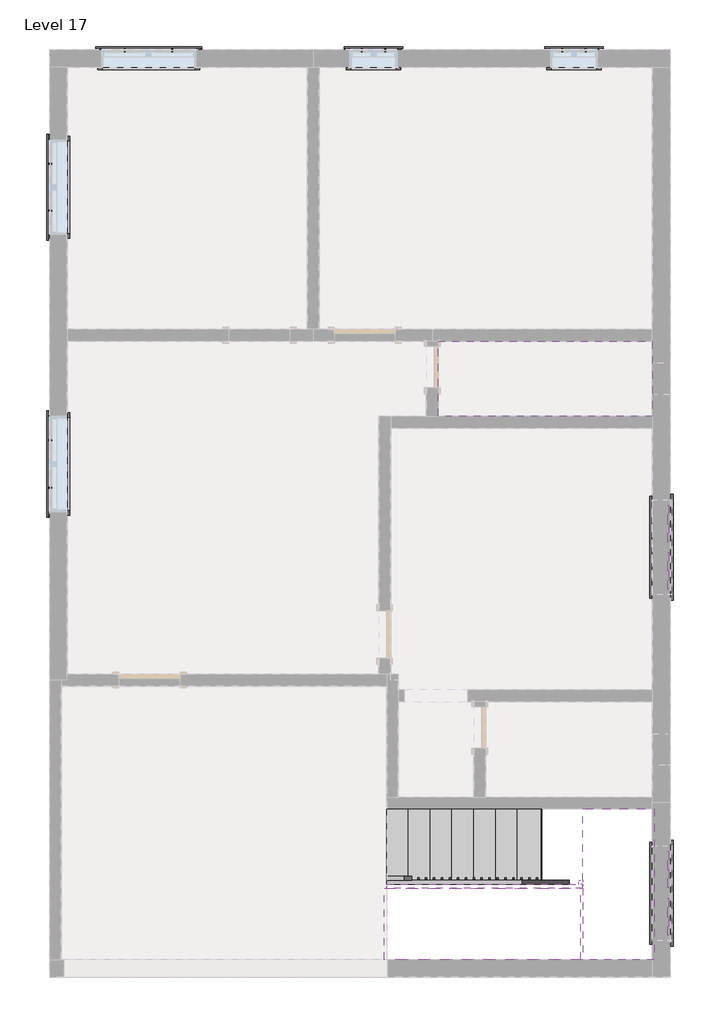
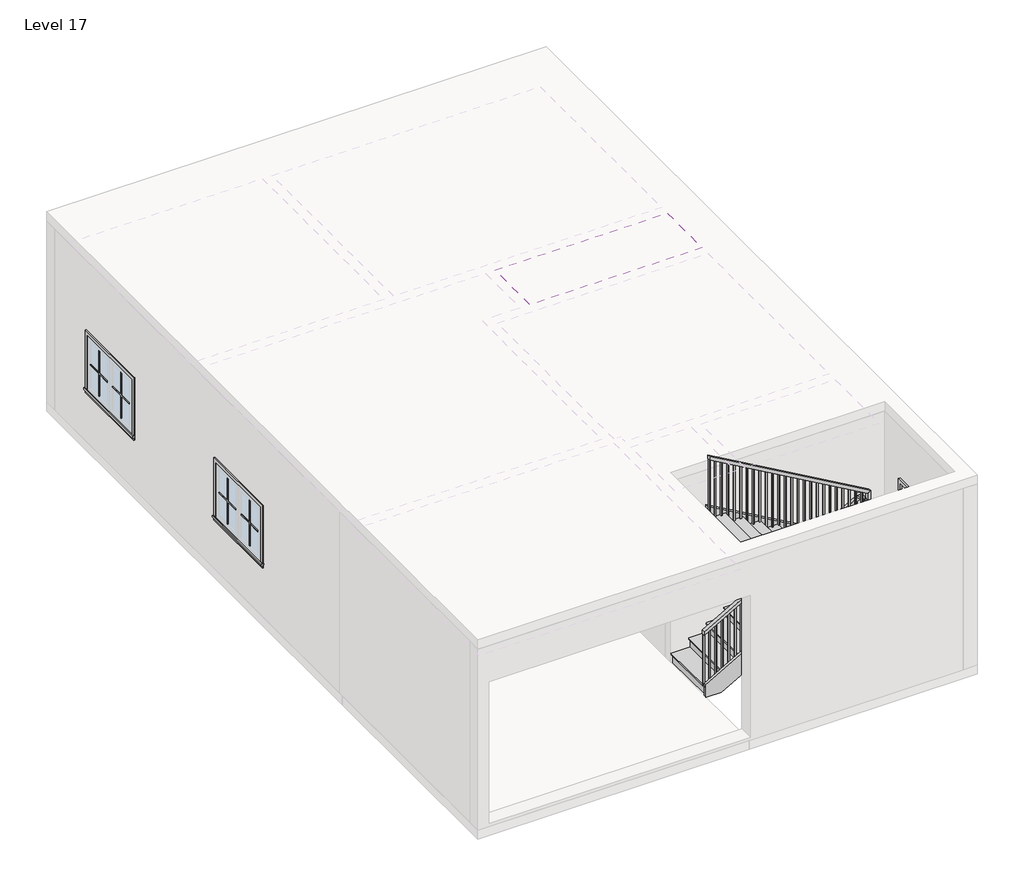
# One storey, part 2 of 2: 44 proxies, 3 members, 2 stair flights, 1 covering, 1 railing, 1 slab.
"""IFC4 building model written with IfcOpenShell, lengths in millimetres."""

from ifc_helpers import new_model, si_unit, frame, origin, place, context, project, spatial, polyline, outline, extrude, faceted_brep, transform, mapped, element, save
from components import muntin_pattern_2x2_muntin_pattern_2x2_2357e71d, muntin_pattern_2x2_muntin_pattern_2x2_302d8f29, muntin_pattern_2x2_muntin_pattern_2x2_53152e2c, muntin_pattern_2x2_muntin_pattern_2x2_e8f3e573, trim_window_exterior_flat_with_sill_c4e67c73, trim_window_exterior_flat_with_sill_a665a915, trim_window_interior_flat_picture_frame_cf1733af, trim_window_interior_flat_picture_frame_d485c387, non_monolithic_landing_9ec975f3, stair_flight_228e22e8, stair_flight_e10c2242

model = new_model("IFC4")

# Units and contexts
model_context = context("Model", 3, world=origin())
ifc_project = project(units=[si_unit("LENGTHUNIT", "METRE", prefix="MILLI")], contexts=[model_context])

# Site, building, storey
site = spatial("IfcSite", under=ifc_project)
building = spatial("IfcBuilding", under=site)
storey = spatial("IfcBuildingStorey", under=building, Name="Level 17", Elevation=9601.2)

# Proxies
placement = place(None, origin())
muntin_pattern_2x2_muntin_pattern_2x2_shape = muntin_pattern_2x2_muntin_pattern_2x2_2357e71d(model_context)
element("IfcBuildingElementProxy", 1, Name="Muntin Pattern_2x2 : Muntin Pattern_2x2", ObjectType="Muntin Pattern_2x2 : Muntin Pattern_2x2", at=placement, inside=storey, context=model_context, shape_type="MappedRepresentation", body=[
    mapped(muntin_pattern_2x2_muntin_pattern_2x2_shape, transform((-4942.3279463, 5897.3080275, 10585.45), x_axis=(1.0, 0.0, 0.0), y_axis=(0.0, 1.0, 0.0), z_axis=(0.0, 0.0, 1.0))),
])
element("IfcBuildingElementProxy", 2, Name="Muntin Pattern_2x2 : Muntin Pattern_2x2", ObjectType="Muntin Pattern_2x2 : Muntin Pattern_2x2", at=placement, inside=storey, context=model_context, shape_type="MappedRepresentation", body=[
    mapped(muntin_pattern_2x2_muntin_pattern_2x2_shape, transform((-5899.5904463, 3838.3205275, 10585.45), x_axis=(0.0, 1.0, 0.0), y_axis=(-1.0, 0.0, 0.0), z_axis=(0.0, 0.0, 1.0))),
])
element("IfcBuildingElementProxy", 3, Name="Muntin Pattern_2x2 : Muntin Pattern_2x2", ObjectType="Muntin Pattern_2x2 : Muntin Pattern_2x2", at=placement, inside=storey, context=model_context, shape_type="MappedRepresentation", body=[
    mapped(muntin_pattern_2x2_muntin_pattern_2x2_shape, transform((-5899.5904463, 293.4330275, 10585.45), x_axis=(0.0, 1.0, 0.0), y_axis=(-1.0, 0.0, 0.0), z_axis=(0.0, 0.0, 1.0))),
])
element("IfcBuildingElementProxy", 4, Name="Muntin Pattern_2x2 : Muntin Pattern_2x2", ObjectType="Muntin Pattern_2x2 : Muntin Pattern_2x2", at=placement, inside=storey, context=model_context, shape_type="MappedRepresentation", body=[
    mapped(muntin_pattern_2x2_muntin_pattern_2x2_shape, transform((2031.5595537, -166.9419725, 10890.25), x_axis=(0.0, -1.0, 0.0), y_axis=(1.0, 0.0, 0.0), z_axis=(0.0, 0.0, 1.0))),
])
element("IfcBuildingElementProxy", 5, Name="Muntin Pattern_2x2 : Muntin Pattern_2x2", ObjectType="Muntin Pattern_2x2 : Muntin Pattern_2x2", at=placement, inside=storey, context=model_context, shape_type="MappedRepresentation", body=[
    mapped(muntin_pattern_2x2_muntin_pattern_2x2_shape, transform((2031.5595537, -4599.2419725, 10890.25), x_axis=(0.0, -1.0, 0.0), y_axis=(1.0, 0.0, 0.0), z_axis=(0.0, 0.0, 1.0))),
])
element("IfcBuildingElementProxy", 6, Name="Muntin Pattern_2x2 : Muntin Pattern_2x2", ObjectType="Muntin Pattern_2x2 : Muntin Pattern_2x2", at=placement, inside=storey, context=model_context, shape_type="MappedRepresentation", body=[
    mapped(muntin_pattern_2x2_muntin_pattern_2x2_shape, transform((-4942.3279463, 5897.3080275, 10585.45), x_axis=(1.0, 0.0, 0.0), y_axis=(0.0, 1.0, 0.0), z_axis=(0.0, 0.0, 1.0))),
])
element("IfcBuildingElementProxy", 7, Name="Muntin Pattern_2x2 : Muntin Pattern_2x2", ObjectType="Muntin Pattern_2x2 : Muntin Pattern_2x2", at=placement, inside=storey, context=model_context, shape_type="MappedRepresentation", body=[
    mapped(muntin_pattern_2x2_muntin_pattern_2x2_shape, transform((2031.5595537, -4599.2419725, 10890.25), x_axis=(0.0, -1.0, 0.0), y_axis=(1.0, 0.0, 0.0), z_axis=(0.0, 0.0, 1.0))),
])
muntin_pattern_2x2_muntin_pattern_2x2_2_shape = muntin_pattern_2x2_muntin_pattern_2x2_302d8f29(model_context)
element("IfcBuildingElementProxy", 8, Name="Muntin Pattern_2x2 : Muntin Pattern_2x2", ObjectType="Muntin Pattern_2x2 : Muntin Pattern_2x2", at=placement, inside=storey, context=model_context, shape_type="MappedRepresentation", body=[
    mapped(muntin_pattern_2x2_muntin_pattern_2x2_2_shape, transform((-4335.9029463, 5897.3080275, 10585.45), x_axis=(-1.0, 0.0, 0.0), y_axis=(0.0, -1.0, 0.0), z_axis=(0.0, 0.0, 1.0))),
])
element("IfcBuildingElementProxy", 9, Name="Muntin Pattern_2x2 : Muntin Pattern_2x2", ObjectType="Muntin Pattern_2x2 : Muntin Pattern_2x2", at=placement, inside=storey, context=model_context, shape_type="MappedRepresentation", body=[
    mapped(muntin_pattern_2x2_muntin_pattern_2x2_2_shape, transform((-5899.5904463, 4444.7455275, 10585.45), x_axis=(0.0, -1.0, 0.0), y_axis=(1.0, 0.0, 0.0), z_axis=(0.0, 0.0, 1.0))),
])
element("IfcBuildingElementProxy", 10, Name="Muntin Pattern_2x2 : Muntin Pattern_2x2", ObjectType="Muntin Pattern_2x2 : Muntin Pattern_2x2", at=placement, inside=storey, context=model_context, shape_type="MappedRepresentation", body=[
    mapped(muntin_pattern_2x2_muntin_pattern_2x2_2_shape, transform((-5899.5904463, 899.8580275, 10585.45), x_axis=(0.0, -1.0, 0.0), y_axis=(1.0, 0.0, 0.0), z_axis=(0.0, 0.0, 1.0))),
])
element("IfcBuildingElementProxy", 11, Name="Muntin Pattern_2x2 : Muntin Pattern_2x2", ObjectType="Muntin Pattern_2x2 : Muntin Pattern_2x2", at=placement, inside=storey, context=model_context, shape_type="MappedRepresentation", body=[
    mapped(muntin_pattern_2x2_muntin_pattern_2x2_2_shape, transform((2031.5595537, -773.3669725, 10890.25), x_axis=(0.0, 1.0, 0.0), y_axis=(-1.0, 0.0, 0.0), z_axis=(0.0, 0.0, 1.0))),
])
element("IfcBuildingElementProxy", 12, Name="Muntin Pattern_2x2 : Muntin Pattern_2x2", ObjectType="Muntin Pattern_2x2 : Muntin Pattern_2x2", at=placement, inside=storey, context=model_context, shape_type="MappedRepresentation", body=[
    mapped(muntin_pattern_2x2_muntin_pattern_2x2_2_shape, transform((2031.5595537, -5205.6669725, 10890.25), x_axis=(0.0, 1.0, 0.0), y_axis=(-1.0, 0.0, 0.0), z_axis=(0.0, 0.0, 1.0))),
])
element("IfcBuildingElementProxy", 13, Name="Muntin Pattern_2x2 : Muntin Pattern_2x2", ObjectType="Muntin Pattern_2x2 : Muntin Pattern_2x2", at=placement, inside=storey, context=model_context, shape_type="MappedRepresentation", body=[
    mapped(muntin_pattern_2x2_muntin_pattern_2x2_2_shape, transform((-4335.9029463, 5897.3080275, 10585.45), x_axis=(-1.0, 0.0, 0.0), y_axis=(0.0, -1.0, 0.0), z_axis=(0.0, 0.0, 1.0))),
])
element("IfcBuildingElementProxy", 14, Name="Muntin Pattern_2x2 : Muntin Pattern_2x2", ObjectType="Muntin Pattern_2x2 : Muntin Pattern_2x2", at=placement, inside=storey, context=model_context, shape_type="MappedRepresentation", body=[
    mapped(muntin_pattern_2x2_muntin_pattern_2x2_2_shape, transform((2031.5595537, -5205.6669725, 10890.25), x_axis=(0.0, 1.0, 0.0), y_axis=(-1.0, 0.0, 0.0), z_axis=(0.0, 0.0, 1.0))),
])
muntin_pattern_2x2_muntin_pattern_2x2_3_shape = muntin_pattern_2x2_muntin_pattern_2x2_53152e2c(model_context)
element("IfcBuildingElementProxy", 15, Name="Muntin Pattern_2x2 : Muntin Pattern_2x2", ObjectType="Muntin Pattern_2x2 : Muntin Pattern_2x2", at=placement, inside=storey, context=model_context, shape_type="MappedRepresentation", body=[
    mapped(muntin_pattern_2x2_muntin_pattern_2x2_3_shape, transform((-1907.0279463, 5897.3080275, 10585.45), x_axis=(1.0, 0.0, 0.0), y_axis=(0.0, 1.0, 0.0), z_axis=(0.0, 0.0, 1.0))),
])
element("IfcBuildingElementProxy", 16, Name="Muntin Pattern_2x2 : Muntin Pattern_2x2", ObjectType="Muntin Pattern_2x2 : Muntin Pattern_2x2", at=placement, inside=storey, context=model_context, shape_type="MappedRepresentation", body=[
    mapped(muntin_pattern_2x2_muntin_pattern_2x2_3_shape, transform((658.3720537, 5897.3080275, 10585.45), x_axis=(1.0, 0.0, 0.0), y_axis=(0.0, 1.0, 0.0), z_axis=(0.0, 0.0, 1.0))),
])
element("IfcBuildingElementProxy", 17, Name="Muntin Pattern_2x2 : Muntin Pattern_2x2", ObjectType="Muntin Pattern_2x2 : Muntin Pattern_2x2", at=placement, inside=storey, context=model_context, shape_type="MappedRepresentation", body=[
    mapped(muntin_pattern_2x2_muntin_pattern_2x2_3_shape, transform((-1907.0279463, 5897.3080275, 10585.45), x_axis=(1.0, 0.0, 0.0), y_axis=(0.0, 1.0, 0.0), z_axis=(0.0, 0.0, 1.0))),
])
element("IfcBuildingElementProxy", 18, Name="Muntin Pattern_2x2 : Muntin Pattern_2x2", ObjectType="Muntin Pattern_2x2 : Muntin Pattern_2x2", at=placement, inside=storey, context=model_context, shape_type="MappedRepresentation", body=[
    mapped(muntin_pattern_2x2_muntin_pattern_2x2_3_shape, transform((658.3720537, 5897.3080275, 10585.45), x_axis=(1.0, 0.0, 0.0), y_axis=(0.0, 1.0, 0.0), z_axis=(0.0, 0.0, 1.0))),
])
muntin_pattern_2x2_muntin_pattern_2x2_4_shape = muntin_pattern_2x2_muntin_pattern_2x2_e8f3e573(model_context)
element("IfcBuildingElementProxy", 19, Name="Muntin Pattern_2x2 : Muntin Pattern_2x2", ObjectType="Muntin Pattern_2x2 : Muntin Pattern_2x2", at=placement, inside=storey, context=model_context, shape_type="MappedRepresentation", body=[
    mapped(muntin_pattern_2x2_muntin_pattern_2x2_4_shape, transform((-1605.4029463, 5897.3080275, 10585.45), x_axis=(-1.0, 0.0, 0.0), y_axis=(0.0, -1.0, 0.0), z_axis=(0.0, 0.0, 1.0))),
])
element("IfcBuildingElementProxy", 20, Name="Muntin Pattern_2x2 : Muntin Pattern_2x2", ObjectType="Muntin Pattern_2x2 : Muntin Pattern_2x2", at=placement, inside=storey, context=model_context, shape_type="MappedRepresentation", body=[
    mapped(muntin_pattern_2x2_muntin_pattern_2x2_4_shape, transform((959.9970537, 5897.3080275, 10585.45), x_axis=(-1.0, 0.0, 0.0), y_axis=(0.0, -1.0, 0.0), z_axis=(0.0, 0.0, 1.0))),
])
element("IfcBuildingElementProxy", 21, Name="Muntin Pattern_2x2 : Muntin Pattern_2x2", ObjectType="Muntin Pattern_2x2 : Muntin Pattern_2x2", at=placement, inside=storey, context=model_context, shape_type="MappedRepresentation", body=[
    mapped(muntin_pattern_2x2_muntin_pattern_2x2_4_shape, transform((-1605.4029463, 5897.3080275, 10585.45), x_axis=(-1.0, 0.0, 0.0), y_axis=(0.0, -1.0, 0.0), z_axis=(0.0, 0.0, 1.0))),
])
element("IfcBuildingElementProxy", 22, Name="Muntin Pattern_2x2 : Muntin Pattern_2x2", ObjectType="Muntin Pattern_2x2 : Muntin Pattern_2x2", at=placement, inside=storey, context=model_context, shape_type="MappedRepresentation", body=[
    mapped(muntin_pattern_2x2_muntin_pattern_2x2_4_shape, transform((959.9970537, 5897.3080275, 10585.45), x_axis=(-1.0, 0.0, 0.0), y_axis=(0.0, -1.0, 0.0), z_axis=(0.0, 0.0, 1.0))),
])
trim_window_exterior_flat_with_sill_shape = trim_window_exterior_flat_with_sill_c4e67c73(model_context)
element("IfcBuildingElementProxy", 23, Name="Trim-Window-Exterior-Flat : with Sill", ObjectType="Trim-Window-Exterior-Flat : with Sill", at=placement, inside=storey, context=model_context, shape_type="MappedRepresentation", body=[
    mapped(trim_window_exterior_flat_with_sill_shape, transform((-4639.1154463, 5906.8330275, 11430.0), x_axis=(-1.0, 0.0, 0.0), y_axis=(0.0, 0.0, 1.0), z_axis=(0.0, 1.0, 0.0))),
])
element("IfcBuildingElementProxy", 24, Name="Trim-Window-Exterior-Flat : with Sill", ObjectType="Trim-Window-Exterior-Flat : with Sill", at=placement, inside=storey, context=model_context, shape_type="MappedRepresentation", body=[
    mapped(trim_window_exterior_flat_with_sill_shape, transform((-5909.1154463, 4141.5330275, 11430.0), x_axis=(0.0, -1.0, 0.0), y_axis=(0.0, 0.0, 1.0), z_axis=(-1.0, 0.0, 0.0))),
])
element("IfcBuildingElementProxy", 25, Name="Trim-Window-Exterior-Flat : with Sill", ObjectType="Trim-Window-Exterior-Flat : with Sill", at=placement, inside=storey, context=model_context, shape_type="MappedRepresentation", body=[
    mapped(trim_window_exterior_flat_with_sill_shape, transform((-5909.1154463, 596.6455275, 11430.0), x_axis=(0.0, -1.0, 0.0), y_axis=(0.0, 0.0, 1.0), z_axis=(-1.0, 0.0, 0.0))),
])
element("IfcBuildingElementProxy", 26, Name="Trim-Window-Exterior-Flat : with Sill", ObjectType="Trim-Window-Exterior-Flat : with Sill", at=placement, inside=storey, context=model_context, shape_type="MappedRepresentation", body=[
    mapped(trim_window_exterior_flat_with_sill_shape, transform((2041.0845537, -470.1544725, 11734.8), x_axis=(0.0, 1.0, 0.0), y_axis=(0.0, 0.0, 1.0), z_axis=(1.0, 0.0, 0.0))),
])
element("IfcBuildingElementProxy", 27, Name="Trim-Window-Exterior-Flat : with Sill", ObjectType="Trim-Window-Exterior-Flat : with Sill", at=placement, inside=storey, context=model_context, shape_type="MappedRepresentation", body=[
    mapped(trim_window_exterior_flat_with_sill_shape, transform((2041.0845537, -4902.4544725, 11734.8), x_axis=(0.0, 1.0, 0.0), y_axis=(0.0, 0.0, 1.0), z_axis=(1.0, 0.0, 0.0))),
])
element("IfcBuildingElementProxy", 28, Name="Trim-Window-Exterior-Flat : with Sill", ObjectType="Trim-Window-Exterior-Flat : with Sill", at=placement, inside=storey, context=model_context, shape_type="MappedRepresentation", body=[
    mapped(trim_window_exterior_flat_with_sill_shape, transform((-4639.1154463, 5906.8330275, 11430.0), x_axis=(-1.0, 0.0, 0.0), y_axis=(0.0, 0.0, 1.0), z_axis=(0.0, 1.0, 0.0))),
])
element("IfcBuildingElementProxy", 29, Name="Trim-Window-Exterior-Flat : with Sill", ObjectType="Trim-Window-Exterior-Flat : with Sill", at=placement, inside=storey, context=model_context, shape_type="MappedRepresentation", body=[
    mapped(trim_window_exterior_flat_with_sill_shape, transform((2041.0845537, -4902.4544725, 11734.8), x_axis=(0.0, 1.0, 0.0), y_axis=(0.0, 0.0, 1.0), z_axis=(1.0, 0.0, 0.0))),
])
trim_window_exterior_flat_with_sill_2_shape = trim_window_exterior_flat_with_sill_a665a915(model_context)
element("IfcBuildingElementProxy", 30, Name="Trim-Window-Exterior-Flat : with Sill", ObjectType="Trim-Window-Exterior-Flat : with Sill", at=placement, inside=storey, context=model_context, shape_type="MappedRepresentation", body=[
    mapped(trim_window_exterior_flat_with_sill_2_shape, transform((-1756.2154463, 5906.8330275, 11430.0), x_axis=(-1.0, 0.0, 0.0), y_axis=(0.0, 0.0, 1.0), z_axis=(0.0, 1.0, 0.0))),
])
element("IfcBuildingElementProxy", 31, Name="Trim-Window-Exterior-Flat : with Sill", ObjectType="Trim-Window-Exterior-Flat : with Sill", at=placement, inside=storey, context=model_context, shape_type="MappedRepresentation", body=[
    mapped(trim_window_exterior_flat_with_sill_2_shape, transform((809.1845537, 5906.8330275, 11430.0), x_axis=(-1.0, 0.0, 0.0), y_axis=(0.0, 0.0, 1.0), z_axis=(0.0, 1.0, 0.0))),
])
element("IfcBuildingElementProxy", 32, Name="Trim-Window-Exterior-Flat : with Sill", ObjectType="Trim-Window-Exterior-Flat : with Sill", at=placement, inside=storey, context=model_context, shape_type="MappedRepresentation", body=[
    mapped(trim_window_exterior_flat_with_sill_2_shape, transform((-1756.2154463, 5906.8330275, 11430.0), x_axis=(-1.0, 0.0, 0.0), y_axis=(0.0, 0.0, 1.0), z_axis=(0.0, 1.0, 0.0))),
])
element("IfcBuildingElementProxy", 33, Name="Trim-Window-Exterior-Flat : with Sill", ObjectType="Trim-Window-Exterior-Flat : with Sill", at=placement, inside=storey, context=model_context, shape_type="MappedRepresentation", body=[
    mapped(trim_window_exterior_flat_with_sill_2_shape, transform((809.1845537, 5906.8330275, 11430.0), x_axis=(-1.0, 0.0, 0.0), y_axis=(0.0, 0.0, 1.0), z_axis=(0.0, 1.0, 0.0))),
])
trim_window_interior_flat_picture_frame_shape = trim_window_interior_flat_picture_frame_cf1733af(model_context)
element("IfcBuildingElementProxy", 34, Name="Trim-Window-Interior-Flat : Picture Frame", ObjectType="Trim-Window-Interior-Flat : Picture Frame", at=placement, inside=storey, context=model_context, shape_type="MappedRepresentation", body=[
    mapped(trim_window_interior_flat_picture_frame_shape, transform((-4639.1154463, 5678.2330275, 11430.0), x_axis=(1.0, 0.0, 0.0), y_axis=(0.0, 0.0, 1.0), z_axis=(0.0, -1.0, 0.0))),
])
element("IfcBuildingElementProxy", 35, Name="Trim-Window-Interior-Flat : Picture Frame", ObjectType="Trim-Window-Interior-Flat : Picture Frame", at=placement, inside=storey, context=model_context, shape_type="MappedRepresentation", body=[
    mapped(trim_window_interior_flat_picture_frame_shape, transform((-5680.5154463, 4141.5330275, 11430.0), x_axis=(0.0, 1.0, 0.0), y_axis=(0.0, 0.0, 1.0), z_axis=(1.0, 0.0, 0.0))),
])
element("IfcBuildingElementProxy", 36, Name="Trim-Window-Interior-Flat : Picture Frame", ObjectType="Trim-Window-Interior-Flat : Picture Frame", at=placement, inside=storey, context=model_context, shape_type="MappedRepresentation", body=[
    mapped(trim_window_interior_flat_picture_frame_shape, transform((-5680.5154463, 596.6455275, 11430.0), x_axis=(0.0, 1.0, 0.0), y_axis=(0.0, 0.0, 1.0), z_axis=(1.0, 0.0, 0.0))),
])
element("IfcBuildingElementProxy", 37, Name="Trim-Window-Interior-Flat : Picture Frame", ObjectType="Trim-Window-Interior-Flat : Picture Frame", at=placement, inside=storey, context=model_context, shape_type="MappedRepresentation", body=[
    mapped(trim_window_interior_flat_picture_frame_shape, transform((1812.4845537, -470.1544725, 11734.8), x_axis=(0.0, -1.0, 0.0), y_axis=(0.0, 0.0, 1.0), z_axis=(-1.0, 0.0, 0.0))),
])
element("IfcBuildingElementProxy", 38, Name="Trim-Window-Interior-Flat : Picture Frame", ObjectType="Trim-Window-Interior-Flat : Picture Frame", at=placement, inside=storey, context=model_context, shape_type="MappedRepresentation", body=[
    mapped(trim_window_interior_flat_picture_frame_shape, transform((1812.4845537, -4902.4544725, 11734.8), x_axis=(0.0, -1.0, 0.0), y_axis=(0.0, 0.0, 1.0), z_axis=(-1.0, 0.0, 0.0))),
])
element("IfcBuildingElementProxy", 39, Name="Trim-Window-Interior-Flat : Picture Frame", ObjectType="Trim-Window-Interior-Flat : Picture Frame", at=placement, inside=storey, context=model_context, shape_type="MappedRepresentation", body=[
    mapped(trim_window_interior_flat_picture_frame_shape, transform((-4639.1154463, 5678.2330275, 11430.0), x_axis=(1.0, 0.0, 0.0), y_axis=(0.0, 0.0, 1.0), z_axis=(0.0, -1.0, 0.0))),
])
element("IfcBuildingElementProxy", 40, Name="Trim-Window-Interior-Flat : Picture Frame", ObjectType="Trim-Window-Interior-Flat : Picture Frame", at=placement, inside=storey, context=model_context, shape_type="MappedRepresentation", body=[
    mapped(trim_window_interior_flat_picture_frame_shape, transform((1812.4845537, -4902.4544725, 11734.8), x_axis=(0.0, -1.0, 0.0), y_axis=(0.0, 0.0, 1.0), z_axis=(-1.0, 0.0, 0.0))),
])
trim_window_interior_flat_picture_frame_2_shape = trim_window_interior_flat_picture_frame_d485c387(model_context)
element("IfcBuildingElementProxy", 41, Name="Trim-Window-Interior-Flat : Picture Frame", ObjectType="Trim-Window-Interior-Flat : Picture Frame", at=placement, inside=storey, context=model_context, shape_type="MappedRepresentation", body=[
    mapped(trim_window_interior_flat_picture_frame_2_shape, transform((-1756.2154463, 5678.2330275, 11430.0), x_axis=(1.0, 0.0, 0.0), y_axis=(0.0, 0.0, 1.0), z_axis=(0.0, -1.0, 0.0))),
])
element("IfcBuildingElementProxy", 42, Name="Trim-Window-Interior-Flat : Picture Frame", ObjectType="Trim-Window-Interior-Flat : Picture Frame", at=placement, inside=storey, context=model_context, shape_type="MappedRepresentation", body=[
    mapped(trim_window_interior_flat_picture_frame_2_shape, transform((809.1845537, 5678.2330275, 11430.0), x_axis=(1.0, 0.0, 0.0), y_axis=(0.0, 0.0, 1.0), z_axis=(0.0, -1.0, 0.0))),
])
element("IfcBuildingElementProxy", 43, Name="Trim-Window-Interior-Flat : Picture Frame", ObjectType="Trim-Window-Interior-Flat : Picture Frame", at=placement, inside=storey, context=model_context, shape_type="MappedRepresentation", body=[
    mapped(trim_window_interior_flat_picture_frame_2_shape, transform((-1756.2154463, 5678.2330275, 11430.0), x_axis=(1.0, 0.0, 0.0), y_axis=(0.0, 0.0, 1.0), z_axis=(0.0, -1.0, 0.0))),
])
element("IfcBuildingElementProxy", 44, Name="Trim-Window-Interior-Flat : Picture Frame", ObjectType="Trim-Window-Interior-Flat : Picture Frame", at=placement, inside=storey, context=model_context, shape_type="MappedRepresentation", body=[
    mapped(trim_window_interior_flat_picture_frame_2_shape, transform((809.1845537, 5678.2330275, 11430.0), x_axis=(1.0, 0.0, 0.0), y_axis=(0.0, 0.0, 1.0), z_axis=(0.0, -1.0, 0.0))),
])

# Covering
element("IfcCovering", 45, ObjectType="2' x 4' ACT System", at=placement, inside=storey, context=model_context, shape_type="SweptSolid", body=[
    extrude(outline(polyline([(-930.7154463, 2171.4455275), (1812.4845537, 2171.4455275), (1812.4845537, 1206.2455275), (-930.7154463, 1206.2455275), (-930.7154463, 2171.4455275)])), frame((0.0, 0.0, 12344.4), z_axis=(0.0, 0.0, 1.0), x_axis=(1.0, 0.0, 0.0)), (0.0, 0.0, 1.0), 57.15),
])

# Members
element("IfcMember", 46, ObjectType="Stringer - 2\" Width", at=placement, inside=storey, context=model_context, shape_type="SweptSolid", body=[
    extrude(outline(polyline([(9810.2890626, -1591.1154463), (9601.2, -1591.1154463), (9601.2, -1342.8974141), (10870.124218, 872.6845537), (11221.3745172, 872.6845537), (9810.2890626, -1591.1154463)])), frame((0.0, -4788.1544725, 0.0), z_axis=(0.0, 1.0, 0.0), x_axis=(0.0, 0.0, 1.0)), (0.0, 0.0, 1.0), 50.8),
])
element("IfcMember", 47, ObjectType="Stringer - 2\" Width", at=placement, inside=storey, context=model_context, shape_type="SweptSolid", body=[
    extrude(outline(polyline([(11059.2387634, 923.4845537), (11410.4890626, 923.4845537), (12850.6690626, -1591.1154463), (12499.4187634, -1591.1154463), (11059.2387634, 923.4845537)])), frame((0.0, -4838.9544725, 0.0), z_axis=(0.0, 1.0, 0.0), x_axis=(0.0, 0.0, 1.0)), (0.0, 0.0, 1.0), 50.8),
])
element("IfcMember", 48, ObjectType="Stringer - 2\" Width", at=placement, inside=storey, context=model_context, shape_type="SweptSolid", body=[
    extrude(outline(polyline([(872.6845537, -4737.3544725), (923.4845537, -4737.3544725), (923.4845537, -4788.1544725), (872.6845537, -4788.1544725), (872.6845537, -4737.3544725)])), frame((0.0, 0.0, 10972.8), z_axis=(0.0, 0.0, 1.0), x_axis=(1.0, 0.0, 0.0)), (0.0, 0.0, 1.0), 304.8),
])

# Railing
element("IfcRailing", 49, ObjectType="Handrail - Rectangular", at=placement, inside=storey, context=model_context, shape_type="SolidModel", body=[
    faceted_brep([(-1591.1154463, -4686.5544725, 10675.62), (-1591.1154463, -4686.5544725, 10617.0782835), (-1591.1154463, -4737.3544725, 10617.0782835), (-1591.1154463, -4737.3544725, 10675.62), (847.2845537, -4686.5544725, 12072.1581818), (898.0845537, -4686.5544725, 12042.7110107), (898.0845537, -4737.3544725, 12042.7110107), (847.2845537, -4737.3544725, 12072.1581818), (847.2845537, -4686.5544725, 12115.8), (898.0845537, -4686.5544725, 12065.0), (898.0845537, -4737.3544725, 12065.0), (847.2845537, -4737.3544725, 12115.8), (974.2845537, -4686.5544725, 12115.8), (974.2845537, -4686.5544725, 12065.0), (923.4845537, -4737.3544725, 12065.0), (923.4845537, -4737.3544725, 12115.8), (974.2845537, -4813.5544725, 12115.8), (974.2845537, -4813.5544725, 12065.0), (923.4845537, -4813.5544725, 12065.0), (923.4845537, -4813.5544725, 12115.8), (974.2845537, -4838.9544725, 12115.8), (923.4845537, -4838.9544725, 12115.8), (923.4845537, -4889.7544725, 12065.0), (974.2845537, -4889.7544725, 12065.0)], [[[0, 1, 2, 3]], [[1, 0, 4, 5]], [[2, 1, 5, 6]], [[3, 2, 6, 7]], [[0, 3, 7, 4]], [[5, 4, 8, 9]], [[6, 5, 9, 10]], [[7, 6, 10, 11]], [[4, 7, 11, 8]], [[9, 8, 12, 13]], [[10, 9, 13, 14]], [[11, 10, 14, 15]], [[8, 11, 15, 12]], [[13, 12, 16, 17]], [[14, 13, 17, 18]], [[15, 14, 18, 19]], [[12, 15, 19, 16]], [[20, 21, 22, 23]], [[17, 16, 20, 23]], [[18, 17, 23, 22]], [[19, 18, 22, 21]], [[16, 19, 21, 20]]]),
    faceted_brep([(974.2845537, -4838.9544725, 12115.8), (974.2845537, -4889.7544725, 12065.0), (923.4845537, -4889.7544725, 12065.0), (923.4845537, -4838.9544725, 12115.8), (974.2845537, -4838.9544725, 12246.7254545), (923.4845537, -4838.9544725, 12217.2782835), (923.4845537, -4889.7544725, 12217.2782835), (974.2845537, -4889.7544725, 12246.7254545)], [[[0, 1, 2, 3]], [[4, 5, 6, 7]], [[1, 0, 4, 7]], [[2, 1, 7, 6]], [[3, 2, 6, 5]], [[0, 3, 5, 4]]]),
    faceted_brep([(974.2845537, -4889.7544725, 12246.7254545), (923.4845537, -4889.7544725, 12217.2782835), (923.4845537, -4838.9544725, 12217.2782835), (974.2845537, -4838.9544725, 12246.7254545), (-1591.1154463, -4889.7544725, 13716.0), (-1591.1154463, -4838.9544725, 13716.0), (-1591.1154463, -4838.9544725, 13657.4582835), (-1591.1154463, -4889.7544725, 13657.4582835)], [[[0, 1, 2, 3]], [[4, 5, 6, 7]], [[1, 0, 4, 7]], [[2, 1, 7, 6]], [[3, 2, 6, 5]], [[0, 3, 5, 4]]]),
    extrude(outline(polyline([(13593.8139653, -1479.9904463), (13604.7244198, -1499.0404463), (12641.58, -1499.0404463), (12641.58, -1479.9904463), (13593.8139653, -1479.9904463)])), frame((0.0, -4873.8794725, 0.0), z_axis=(0.0, 1.0, 0.0), x_axis=(0.0, 0.0, 1.0)), (0.0, 0.0, 1.0), 19.05),
    extrude(outline(polyline([(13535.6248744, -1378.3904463), (13546.5353289, -1397.4404463), (12641.58, -1397.4404463), (12641.58, -1378.3904463), (13535.6248744, -1378.3904463)])), frame((0.0, -4873.8794725, 0.0), z_axis=(0.0, 1.0, 0.0), x_axis=(0.0, 0.0, 1.0)), (0.0, 0.0, 1.0), 19.05),
    extrude(outline(polyline([(13477.4357835, -1276.7904463), (13488.346238, -1295.8404463), (12481.56, -1295.8404463), (12481.56, -1276.7904463), (13477.4357835, -1276.7904463)])), frame((0.0, -4873.8794725, 0.0), z_axis=(0.0, 1.0, 0.0), x_axis=(0.0, 0.0, 1.0)), (0.0, 0.0, 1.0), 19.05),
    extrude(outline(polyline([(13419.2466926, -1175.1904463), (13430.1571471, -1194.2404463), (12481.56, -1194.2404463), (12481.56, -1175.1904463), (13419.2466926, -1175.1904463)])), frame((0.0, -4873.8794725, 0.0), z_axis=(0.0, 1.0, 0.0), x_axis=(0.0, 0.0, 1.0)), (0.0, 0.0, 1.0), 19.05),
    extrude(outline(polyline([(13361.0576016, -1073.5904463), (13371.9680562, -1092.6404463), (12481.56, -1092.6404463), (12481.56, -1073.5904463), (13361.0576016, -1073.5904463)])), frame((0.0, -4873.8794725, 0.0), z_axis=(0.0, 1.0, 0.0), x_axis=(0.0, 0.0, 1.0)), (0.0, 0.0, 1.0), 19.05),
    extrude(outline(polyline([(13302.8685107, -971.9904463), (13313.7789653, -991.0404463), (12321.54, -991.0404463), (12321.54, -971.9904463), (13302.8685107, -971.9904463)])), frame((0.0, -4873.8794725, 0.0), z_axis=(0.0, 1.0, 0.0), x_axis=(0.0, 0.0, 1.0)), (0.0, 0.0, 1.0), 19.05),
    extrude(outline(polyline([(13244.6794198, -870.3904463), (13255.5898744, -889.4404463), (12321.54, -889.4404463), (12321.54, -870.3904463), (13244.6794198, -870.3904463)])), frame((0.0, -4873.8794725, 0.0), z_axis=(0.0, 1.0, 0.0), x_axis=(0.0, 0.0, 1.0)), (0.0, 0.0, 1.0), 19.05),
    extrude(outline(polyline([(13186.4903289, -768.7904463), (13197.4007835, -787.8404463), (12321.54, -787.8404463), (12321.54, -768.7904463), (13186.4903289, -768.7904463)])), frame((0.0, -4873.8794725, 0.0), z_axis=(0.0, 1.0, 0.0), x_axis=(0.0, 0.0, 1.0)), (0.0, 0.0, 1.0), 19.05),
    extrude(outline(polyline([(13128.301238, -667.1904463), (13139.2116926, -686.2404463), (12161.52, -686.2404463), (12161.52, -667.1904463), (13128.301238, -667.1904463)])), frame((0.0, -4873.8794725, 0.0), z_axis=(0.0, 1.0, 0.0), x_axis=(0.0, 0.0, 1.0)), (0.0, 0.0, 1.0), 19.05),
    extrude(outline(polyline([(13070.1121471, -565.5904463), (13081.0226016, -584.6404463), (12161.52, -584.6404463), (12161.52, -565.5904463), (13070.1121471, -565.5904463)])), frame((0.0, -4873.8794725, 0.0), z_axis=(0.0, 1.0, 0.0), x_axis=(0.0, 0.0, 1.0)), (0.0, 0.0, 1.0), 19.05),
    extrude(outline(polyline([(13011.9230562, -463.9904463), (13022.8335107, -483.0404463), (12161.52, -483.0404463), (12161.52, -463.9904463), (13011.9230562, -463.9904463)])), frame((0.0, -4873.8794725, 0.0), z_axis=(0.0, 1.0, 0.0), x_axis=(0.0, 0.0, 1.0)), (0.0, 0.0, 1.0), 19.05),
    extrude(outline(polyline([(12953.7339653, -362.3904463), (12964.6444198, -381.4404463), (12001.5, -381.4404463), (12001.5, -362.3904463), (12953.7339653, -362.3904463)])), frame((0.0, -4873.8794725, 0.0), z_axis=(0.0, 1.0, 0.0), x_axis=(0.0, 0.0, 1.0)), (0.0, 0.0, 1.0), 19.05),
    extrude(outline(polyline([(12895.5448744, -260.7904463), (12906.4553289, -279.8404463), (12001.5, -279.8404463), (12001.5, -260.7904463), (12895.5448744, -260.7904463)])), frame((0.0, -4873.8794725, 0.0), z_axis=(0.0, 1.0, 0.0), x_axis=(0.0, 0.0, 1.0)), (0.0, 0.0, 1.0), 19.05),
    extrude(outline(polyline([(12837.3557835, -159.1904463), (12848.266238, -178.2404463), (11841.48, -178.2404463), (11841.48, -159.1904463), (12837.3557835, -159.1904463)])), frame((0.0, -4873.8794725, 0.0), z_axis=(0.0, 1.0, 0.0), x_axis=(0.0, 0.0, 1.0)), (0.0, 0.0, 1.0), 19.05),
    extrude(outline(polyline([(12779.1666926, -57.5904463), (12790.0771471, -76.6404463), (11841.48, -76.6404463), (11841.48, -57.5904463), (12779.1666926, -57.5904463)])), frame((0.0, -4873.8794725, 0.0), z_axis=(0.0, 1.0, 0.0), x_axis=(0.0, 0.0, 1.0)), (0.0, 0.0, 1.0), 19.05),
    extrude(outline(polyline([(12720.9776016, 44.0095537), (12731.8880562, 24.9595537), (11841.48, 24.9595537), (11841.48, 44.0095537), (12720.9776016, 44.0095537)])), frame((0.0, -4873.8794725, 0.0), z_axis=(0.0, 1.0, 0.0), x_axis=(0.0, 0.0, 1.0)), (0.0, 0.0, 1.0), 19.05),
    extrude(outline(polyline([(12662.7885107, 145.6095537), (12673.6989653, 126.5595537), (11681.46, 126.5595537), (11681.46, 145.6095537), (12662.7885107, 145.6095537)])), frame((0.0, -4873.8794725, 0.0), z_axis=(0.0, 1.0, 0.0), x_axis=(0.0, 0.0, 1.0)), (0.0, 0.0, 1.0), 19.05),
    extrude(outline(polyline([(12604.5994198, 247.2095537), (12615.5098744, 228.1595537), (11681.46, 228.1595537), (11681.46, 247.2095537), (12604.5994198, 247.2095537)])), frame((0.0, -4873.8794725, 0.0), z_axis=(0.0, 1.0, 0.0), x_axis=(0.0, 0.0, 1.0)), (0.0, 0.0, 1.0), 19.05),
    extrude(outline(polyline([(12546.4103289, 348.8095537), (12557.3207835, 329.7595537), (11681.46, 329.7595537), (11681.46, 348.8095537), (12546.4103289, 348.8095537)])), frame((0.0, -4873.8794725, 0.0), z_axis=(0.0, 1.0, 0.0), x_axis=(0.0, 0.0, 1.0)), (0.0, 0.0, 1.0), 19.05),
    extrude(outline(polyline([(12488.221238, 450.4095537), (12499.1316926, 431.3595537), (11521.44, 431.3595537), (11521.44, 450.4095537), (12488.221238, 450.4095537)])), frame((0.0, -4873.8794725, 0.0), z_axis=(0.0, 1.0, 0.0), x_axis=(0.0, 0.0, 1.0)), (0.0, 0.0, 1.0), 19.05),
    extrude(outline(polyline([(12430.0321471, 552.0095537), (12440.9426016, 532.9595537), (11521.44, 532.9595537), (11521.44, 552.0095537), (12430.0321471, 552.0095537)])), frame((0.0, -4873.8794725, 0.0), z_axis=(0.0, 1.0, 0.0), x_axis=(0.0, 0.0, 1.0)), (0.0, 0.0, 1.0), 19.05),
    extrude(outline(polyline([(12371.8430562, 653.6095537), (12382.7535107, 634.5595537), (11521.44, 634.5595537), (11521.44, 653.6095537), (12371.8430562, 653.6095537)])), frame((0.0, -4873.8794725, 0.0), z_axis=(0.0, 1.0, 0.0), x_axis=(0.0, 0.0, 1.0)), (0.0, 0.0, 1.0), 19.05),
    extrude(outline(polyline([(12313.6539653, 755.2095537), (12324.5644198, 736.1595537), (11361.42, 736.1595537), (11361.42, 755.2095537), (12313.6539653, 755.2095537)])), frame((0.0, -4873.8794725, 0.0), z_axis=(0.0, 1.0, 0.0), x_axis=(0.0, 0.0, 1.0)), (0.0, 0.0, 1.0), 19.05),
    extrude(outline(polyline([(12255.4648744, 856.8095537), (12266.3753289, 837.7595537), (11361.42, 837.7595537), (11361.42, 856.8095537), (12255.4648744, 856.8095537)])), frame((0.0, -4873.8794725, 0.0), z_axis=(0.0, 1.0, 0.0), x_axis=(0.0, 0.0, 1.0)), (0.0, 0.0, 1.0), 19.05),
    extrude(outline(polyline([(939.3595537, -4804.0294725), (958.4095537, -4804.0294725), (958.4095537, -4823.0794725), (939.3595537, -4823.0794725), (939.3595537, -4804.0294725)])), frame((0.0, 0.0, 11201.4), z_axis=(0.0, 0.0, 1.0), x_axis=(1.0, 0.0, 0.0)), (0.0, 0.0, 1.0), 863.6),
    extrude(outline(polyline([(12019.0716926, 856.8095537), (12008.161238, 837.7595537), (11041.38, 837.7595537), (11041.38, 856.8095537), (12019.0716926, 856.8095537)])), frame((0.0, -4721.4794725, 0.0), z_axis=(0.0, 1.0, 0.0), x_axis=(0.0, 0.0, 1.0)), (0.0, 0.0, 1.0), 19.05),
    extrude(outline(polyline([(11960.8826016, 755.2095537), (11949.9721471, 736.1595537), (11041.38, 736.1595537), (11041.38, 755.2095537), (11960.8826016, 755.2095537)])), frame((0.0, -4721.4794725, 0.0), z_axis=(0.0, 1.0, 0.0), x_axis=(0.0, 0.0, 1.0)), (0.0, 0.0, 1.0), 19.05),
    extrude(outline(polyline([(11902.6935107, 653.6095537), (11891.7830562, 634.5595537), (11041.38, 634.5595537), (11041.38, 653.6095537), (11902.6935107, 653.6095537)])), frame((0.0, -4721.4794725, 0.0), z_axis=(0.0, 1.0, 0.0), x_axis=(0.0, 0.0, 1.0)), (0.0, 0.0, 1.0), 19.05),
    extrude(outline(polyline([(11844.5044198, 552.0095537), (11833.5939653, 532.9595537), (10881.36, 532.9595537), (10881.36, 552.0095537), (11844.5044198, 552.0095537)])), frame((0.0, -4721.4794725, 0.0), z_axis=(0.0, 1.0, 0.0), x_axis=(0.0, 0.0, 1.0)), (0.0, 0.0, 1.0), 19.05),
    extrude(outline(polyline([(11786.3153289, 450.4095537), (11775.4048744, 431.3595537), (10881.36, 431.3595537), (10881.36, 450.4095537), (11786.3153289, 450.4095537)])), frame((0.0, -4721.4794725, 0.0), z_axis=(0.0, 1.0, 0.0), x_axis=(0.0, 0.0, 1.0)), (0.0, 0.0, 1.0), 19.05),
    extrude(outline(polyline([(11728.126238, 348.8095537), (11717.2157835, 329.7595537), (10721.34, 329.7595537), (10721.34, 348.8095537), (11728.126238, 348.8095537)])), frame((0.0, -4721.4794725, 0.0), z_axis=(0.0, 1.0, 0.0), x_axis=(0.0, 0.0, 1.0)), (0.0, 0.0, 1.0), 19.05),
    extrude(outline(polyline([(11669.9371471, 247.2095537), (11659.0266926, 228.1595537), (10721.34, 228.1595537), (10721.34, 247.2095537), (11669.9371471, 247.2095537)])), frame((0.0, -4721.4794725, 0.0), z_axis=(0.0, 1.0, 0.0), x_axis=(0.0, 0.0, 1.0)), (0.0, 0.0, 1.0), 19.05),
    extrude(outline(polyline([(11611.7480562, 145.6095537), (11600.8376016, 126.5595537), (10721.34, 126.5595537), (10721.34, 145.6095537), (11611.7480562, 145.6095537)])), frame((0.0, -4721.4794725, 0.0), z_axis=(0.0, 1.0, 0.0), x_axis=(0.0, 0.0, 1.0)), (0.0, 0.0, 1.0), 19.05),
    extrude(outline(polyline([(11553.5589653, 44.0095537), (11542.6485107, 24.9595537), (10561.32, 24.9595537), (10561.32, 44.0095537), (11553.5589653, 44.0095537)])), frame((0.0, -4721.4794725, 0.0), z_axis=(0.0, 1.0, 0.0), x_axis=(0.0, 0.0, 1.0)), (0.0, 0.0, 1.0), 19.05),
    extrude(outline(polyline([(11495.3698744, -57.5904463), (11484.4594198, -76.6404463), (10561.32, -76.6404463), (10561.32, -57.5904463), (11495.3698744, -57.5904463)])), frame((0.0, -4721.4794725, 0.0), z_axis=(0.0, 1.0, 0.0), x_axis=(0.0, 0.0, 1.0)), (0.0, 0.0, 1.0), 19.05),
    extrude(outline(polyline([(11437.1807835, -159.1904463), (11426.2703289, -178.2404463), (10561.32, -178.2404463), (10561.32, -159.1904463), (11437.1807835, -159.1904463)])), frame((0.0, -4721.4794725, 0.0), z_axis=(0.0, 1.0, 0.0), x_axis=(0.0, 0.0, 1.0)), (0.0, 0.0, 1.0), 19.05),
    extrude(outline(polyline([(11378.9916926, -260.7904463), (11368.081238, -279.8404463), (10401.3, -279.8404463), (10401.3, -260.7904463), (11378.9916926, -260.7904463)])), frame((0.0, -4721.4794725, 0.0), z_axis=(0.0, 1.0, 0.0), x_axis=(0.0, 0.0, 1.0)), (0.0, 0.0, 1.0), 19.05),
    extrude(outline(polyline([(11320.8026016, -362.3904463), (11309.8921471, -381.4404463), (10401.3, -381.4404463), (10401.3, -362.3904463), (11320.8026016, -362.3904463)])), frame((0.0, -4721.4794725, 0.0), z_axis=(0.0, 1.0, 0.0), x_axis=(0.0, 0.0, 1.0)), (0.0, 0.0, 1.0), 19.05),
    extrude(outline(polyline([(11262.6135107, -463.9904463), (11251.7030562, -483.0404463), (10401.3, -483.0404463), (10401.3, -463.9904463), (11262.6135107, -463.9904463)])), frame((0.0, -4721.4794725, 0.0), z_axis=(0.0, 1.0, 0.0), x_axis=(0.0, 0.0, 1.0)), (0.0, 0.0, 1.0), 19.05),
    extrude(outline(polyline([(11204.4244198, -565.5904463), (11193.5139653, -584.6404463), (10241.28, -584.6404463), (10241.28, -565.5904463), (11204.4244198, -565.5904463)])), frame((0.0, -4721.4794725, 0.0), z_axis=(0.0, 1.0, 0.0), x_axis=(0.0, 0.0, 1.0)), (0.0, 0.0, 1.0), 19.05),
    extrude(outline(polyline([(11146.2353289, -667.1904463), (11135.3248744, -686.2404463), (10241.28, -686.2404463), (10241.28, -667.1904463), (11146.2353289, -667.1904463)])), frame((0.0, -4721.4794725, 0.0), z_axis=(0.0, 1.0, 0.0), x_axis=(0.0, 0.0, 1.0)), (0.0, 0.0, 1.0), 19.05),
    extrude(outline(polyline([(11088.046238, -768.7904463), (11077.1357835, -787.8404463), (10081.26, -787.8404463), (10081.26, -768.7904463), (11088.046238, -768.7904463)])), frame((0.0, -4721.4794725, 0.0), z_axis=(0.0, 1.0, 0.0), x_axis=(0.0, 0.0, 1.0)), (0.0, 0.0, 1.0), 19.05),
    extrude(outline(polyline([(11029.8571471, -870.3904463), (11018.9466926, -889.4404463), (10081.26, -889.4404463), (10081.26, -870.3904463), (11029.8571471, -870.3904463)])), frame((0.0, -4721.4794725, 0.0), z_axis=(0.0, 1.0, 0.0), x_axis=(0.0, 0.0, 1.0)), (0.0, 0.0, 1.0), 19.05),
    extrude(outline(polyline([(10971.6680562, -971.9904463), (10960.7576016, -991.0404463), (10081.26, -991.0404463), (10081.26, -971.9904463), (10971.6680562, -971.9904463)])), frame((0.0, -4721.4794725, 0.0), z_axis=(0.0, 1.0, 0.0), x_axis=(0.0, 0.0, 1.0)), (0.0, 0.0, 1.0), 19.05),
    extrude(outline(polyline([(10913.4789653, -1073.5904463), (10902.5685107, -1092.6404463), (9921.24, -1092.6404463), (9921.24, -1073.5904463), (10913.4789653, -1073.5904463)])), frame((0.0, -4721.4794725, 0.0), z_axis=(0.0, 1.0, 0.0), x_axis=(0.0, 0.0, 1.0)), (0.0, 0.0, 1.0), 19.05),
    extrude(outline(polyline([(10855.2898744, -1175.1904463), (10844.3794198, -1194.2404463), (9921.24, -1194.2404463), (9921.24, -1175.1904463), (10855.2898744, -1175.1904463)])), frame((0.0, -4721.4794725, 0.0), z_axis=(0.0, 1.0, 0.0), x_axis=(0.0, 0.0, 1.0)), (0.0, 0.0, 1.0), 19.05),
    extrude(outline(polyline([(10797.1007835, -1276.7904463), (10786.1903289, -1295.8404463), (9921.24, -1295.8404463), (9921.24, -1276.7904463), (10797.1007835, -1276.7904463)])), frame((0.0, -4721.4794725, 0.0), z_axis=(0.0, 1.0, 0.0), x_axis=(0.0, 0.0, 1.0)), (0.0, 0.0, 1.0), 19.05),
    extrude(outline(polyline([(10738.9116926, -1378.3904463), (10728.001238, -1397.4404463), (9761.22, -1397.4404463), (9761.22, -1378.3904463), (10738.9116926, -1378.3904463)])), frame((0.0, -4721.4794725, 0.0), z_axis=(0.0, 1.0, 0.0), x_axis=(0.0, 0.0, 1.0)), (0.0, 0.0, 1.0), 19.05),
    extrude(outline(polyline([(10680.7226016, -1479.9904463), (10669.8121471, -1499.0404463), (9761.22, -1499.0404463), (9761.22, -1479.9904463), (10680.7226016, -1479.9904463)])), frame((0.0, -4721.4794725, 0.0), z_axis=(0.0, 1.0, 0.0), x_axis=(0.0, 0.0, 1.0)), (0.0, 0.0, 1.0), 19.05),
    extrude(outline(polyline([(939.3595537, -4854.8294725), (958.4095537, -4854.8294725), (958.4095537, -4873.8794725), (939.3595537, -4873.8794725), (939.3595537, -4854.8294725)])), frame((0.0, 0.0, 11201.4), z_axis=(0.0, 0.0, 1.0), x_axis=(1.0, 0.0, 0.0)), (0.0, 0.0, 1.0), 863.6),
    extrude(outline(polyline([(939.3595537, -4721.4794725), (939.3595537, -4702.4294725), (958.4095537, -4702.4294725), (958.4095537, -4721.4794725), (939.3595537, -4721.4794725)])), frame((0.0, 0.0, 11201.4), z_axis=(0.0, 0.0, 1.0), x_axis=(1.0, 0.0, 0.0)), (0.0, 0.0, 1.0), 863.6),
    extrude(outline(polyline([(13646.5478289, -1572.0654463), (13657.4582835, -1591.1154463), (12641.58, -1591.1154463), (12641.58, -1572.0654463), (13646.5478289, -1572.0654463)])), frame((0.0, -4873.8794725, 0.0), z_axis=(0.0, 1.0, 0.0), x_axis=(0.0, 0.0, 1.0)), (0.0, 0.0, 1.0), 19.05),
    extrude(outline(polyline([(10627.988738, -1572.0654463), (10617.0782835, -1591.1154463), (9761.22, -1591.1154463), (9761.22, -1572.0654463), (10627.988738, -1572.0654463)])), frame((0.0, -4721.4794725, 0.0), z_axis=(0.0, 1.0, 0.0), x_axis=(0.0, 0.0, 1.0)), (0.0, 0.0, 1.0), 19.05),
])

# Slab
non_monolithic_landing_shape = non_monolithic_landing_9ec975f3(model_context)
element("IfcSlab", 50, ObjectType="Non-Monolithic Landing", at=placement, inside=storey, context=model_context, shape_type="MappedRepresentation", body=[
    mapped(non_monolithic_landing_shape, transform((0.0, 0.0, 0.0), x_axis=(1.0, 0.0, 0.0), y_axis=(0.0, 1.0, 0.0), z_axis=(0.0, 0.0, 1.0))),
])

# Stair flights
stair_flight_shape = stair_flight_228e22e8(model_context)
element("IfcStairFlight", 51, ObjectType="2\" Tread 1\" Nosing 1/4\" Riser", at=placement, inside=storey, context=model_context, shape_type="MappedRepresentation", body=[
    mapped(stair_flight_shape, transform((0.0, 0.0, 0.0), x_axis=(1.0, 0.0, 0.0), y_axis=(0.0, 1.0, 0.0), z_axis=(0.0, 0.0, 1.0))),
])
stair_flight_2_shape = stair_flight_e10c2242(model_context)
element("IfcStairFlight", 52, ObjectType="2\" Tread 1\" Nosing 1/4\" Riser", at=placement, inside=storey, context=model_context, shape_type="MappedRepresentation", body=[
    mapped(stair_flight_2_shape, transform((0.0, 0.0, 0.0), x_axis=(1.0, 0.0, 0.0), y_axis=(0.0, 1.0, 0.0), z_axis=(0.0, 0.0, 1.0))),
])

save(model, "model.ifc")

# Revit data of these elements
# Type "Muntin Pattern_2x2 : Muntin Pattern_2x2"
#   Width [instance default] = 4' - 0"
#   Thickness = 0' - 0 1/2"
#   Height [instance default] = 4' - 0"
#   Distance = 0' - 0 3/4"
#   Interior Material [instance default] = none
#   Exterior Material [instance default] = none
#   Default Elevation = 0
# Type "Trim-Window-Exterior-Flat : with Sill"
#   Trim Width = 0' - 2 1/4"
#   Trim Thickness_Picture Frame = 0' - 1 1/4"
#   Trim Thickness_with Sill = 0' - 0 3/4"
#   Sill Thickness = 0' - 1 1/4"
#   Opening Width [instance default] = 2' - 0"
#   Opening Height [instance default] = 3' - 0"
#   Default Elevation = 4' - 0"
#   Sill = yes
#   Picture Frame = no
#   Trim Material [instance default] = none
# Type "Trim-Window-Interior-Flat : Picture Frame"
#   Trim Thickness_Picture Frame = 0' - 1 1/4"
#   Trim Width = 0' - 2 1/4"
#   Trim Thickness_with Sill = 0' - 0 3/4"
#   Sill Thickness = 0' - 1 1/4"
#   Opening Width [instance default] = 2' - 0"
#   Opening Height [instance default] = 3' - 0"
#   Default Elevation = 4' - 0"
#   Sill = no
#   Picture Frame = yes
#   Trim Material [instance default] = none
# Type "2' x 4' ACT System"
#   Assembly Code = "C3030210"
#   built-in parameter 1002203 = 1 (stored number, unit not read)
#   built-in parameter 1002202 = 1 (stored number, unit not read)
#   Layers, outside or top first: 0' - 1 5/8" "Default" (function 1); 0' - 0 5/8" "Acoustic Ceiling Tile 24 x 48" (function 5)
# Type "Handrail - Rectangular"
#   Assembly Code = "C2010400"
#   built-in parameter 1008612 = 0.0416667 (stored number, unit not read)
#   built-in parameter 1008611 = 0.0416667 (stored number, unit not read)
#   built-in parameter 1008609 = 0.333333 (stored number, unit not read)
#   built-in parameter 1008604 = 0.166667 (stored number, unit not read)
#   built-in parameter 1008603 = 0.166667 (stored number, unit not read)
#   Railing Height = 3' - 0"
#   built-in parameter 1008630 = 2
#   built-in parameter 1008610 = 2
#   built-in parameter 1008618 = Baluster - Square : 3/4"
# Elements 1, 2, 3, 4, 5, 6, 7, 8, 9, 10, 11, 12, 13, 14 (IfcBuildingElementProxy, "Muntin Pattern_2x2 : Muntin Pattern_2x2")
#   Width = 1' - 6 5/8"
#   Height = 2' - 6 1/2"
#   Interior Material = Wood - Stained
#   Exterior Material = Clad - White
#   Phase Created = New Construction
#   Materials on its faces: "Clad - White", "Wood - Stained"
# Elements 15, 16, 17, 18, 19, 20, 21, 22 (IfcBuildingElementProxy, "Muntin Pattern_2x2 : Muntin Pattern_2x2")
#   Width = 0' - 6 5/8"
#   Height = 2' - 6 1/2"
#   Interior Material = Wood - Stained
#   Exterior Material = Clad - White
#   Phase Created = New Construction
#   Materials on its faces: "Clad - White", "Wood - Stained"
# Elements 23, 24, 25, 26, 27, 28, 29 (IfcBuildingElementProxy, "Trim-Window-Exterior-Flat : with Sill")
#   Opening Width = 4' - 0"
#   Opening Height = 3' - 0"
#   Trim Material = Clad - White
#   Phase Created = New Construction
#   Materials on its faces: "Clad - White"
# Elements 30, 31, 32, 33 (IfcBuildingElementProxy, "Trim-Window-Exterior-Flat : with Sill")
#   Opening Width = 2' - 0"
#   Opening Height = 3' - 0"
#   Trim Material = Clad - White
#   Phase Created = New Construction
#   Materials on its faces: "Clad - White"
# Elements 34, 35, 36, 37, 38, 39, 40 (IfcBuildingElementProxy, "Trim-Window-Interior-Flat : Picture Frame")
#   Opening Width = 4' - 0"
#   Opening Height = 3' - 0"
#   Trim Material = Wood - Stained
#   Phase Created = New Construction
#   Materials on its faces: "Wood - Stained"
# Elements 41, 42, 43, 44 (IfcBuildingElementProxy, "Trim-Window-Interior-Flat : Picture Frame")
#   Opening Width = 2' - 0"
#   Opening Height = 3' - 0"
#   Trim Material = Wood - Stained
#   Phase Created = New Construction
#   Materials on its faces: "Wood - Stained"
# Element 45 (IfcCovering, "2' x 4' ACT System")
#   Height Offset From Level = 9' - 0"
#   Phase Created = New Construction
#   Materials on its faces: "Acoustic Ceiling Tile 24 x 48", "Default"
# Elements 46, 47, 48 (IfcMember, "Stringer - 2\" Width")
#   Phase Created = New Construction
# Element 49 (IfcRailing, "Handrail - Rectangular")
#   Phase Created = New Construction
# Element 50 (IfcSlab, "Non-Monolithic Landing")
#   Phase Created = New Construction
# Elements 51, 52 (IfcStairFlight, "2\" Tread 1\" Nosing 1/4\" Riser")
#   Phase Created = New Construction
# Materials
#   "Default": colour RGB 127 127 127, transparency 0, Cost = 0
#   "Acoustic Ceiling Tile 24 x 48": class "Generic", colour RGB 229 229 229, transparency 0, Description = "Acoustic Ceiling Tile 24 x 48", Cost = 0
#   "Clad - White": class "Wood", colour RGB 242 242 238, transparency 0, Cost = 0
#   "Wood - Stained": class "Wood", colour RGB 224 178 126, transparency 0, Cost = 0
